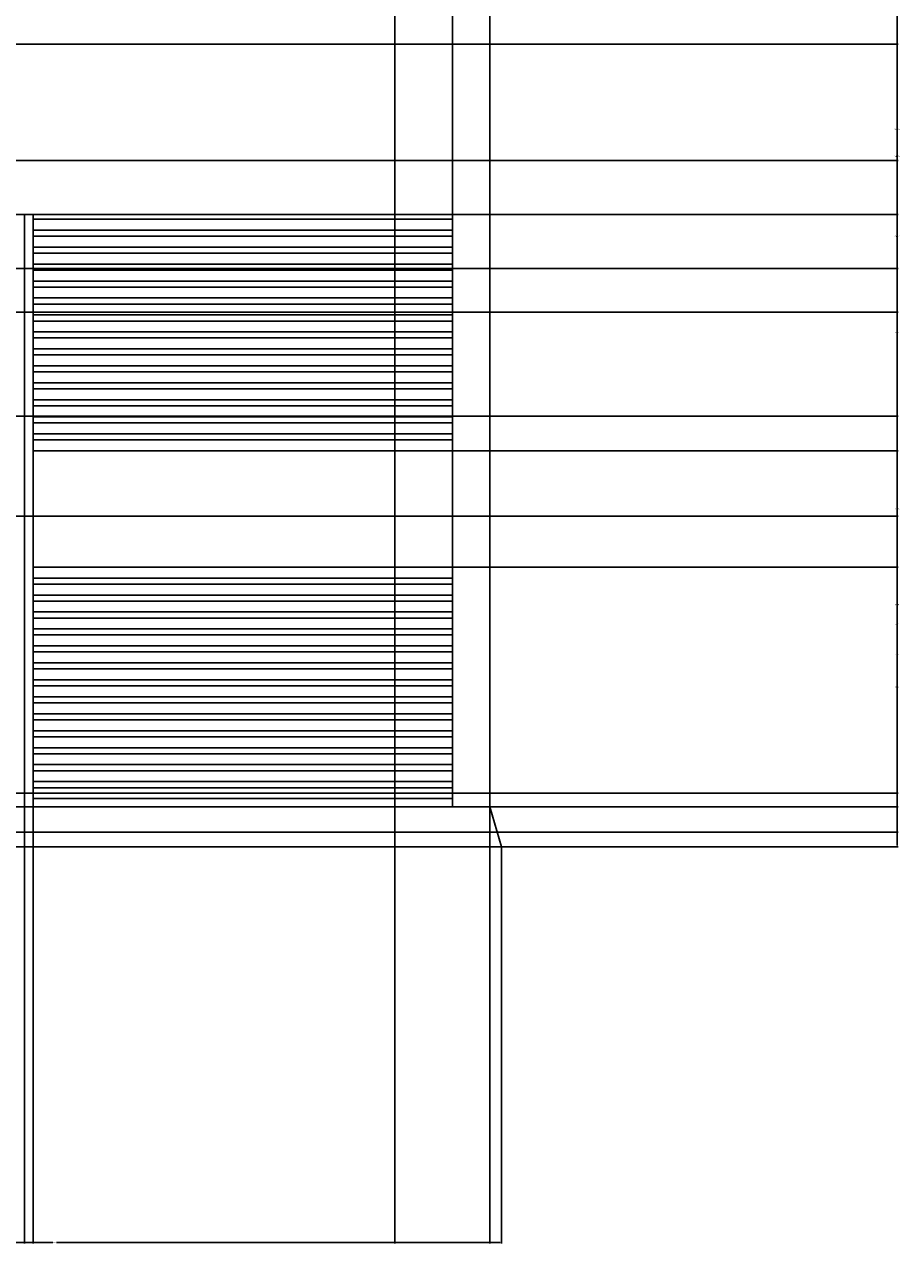
# Model space of a CAD drawing. Units: feet. Extents: x 2193 to 3502, y 890 to 1601.
# Tile 12 of 17: x 3369 to 3502, y 890 to 1076. Entities that reach past the tile are written whole.
import ezdxf

# ---------------------------------------------------------------- set-up
doc = ezdxf.new("R2010")
doc.units = ezdxf.units.FT
doc.layers.add('A-ANNO-DIMS', color=2, linetype='Continuous', lineweight=18)
doc.layers.add('A-ELEV', color=7, linetype='Continuous', lineweight=25)
doc.styles.get("Standard").update_dxf_attribs({"font": 'arial.ttf'})
doc.dimstyles.get("Standard").update_dxf_attribs({"dimtxt": 0.18, "dimasz": 0.18, "dimexe": 0.18, "dimexo": 0.0625, "dimgap": 0.09, "dimtad": 0, "dimtih": 1, "dimtoh": 1, "dimdec": 0, "dimzin": 0, "dimdsep": 46, "dimlunit": 3, "dimtxsty": 'Standard', "dimcen": 0.09, "dimadec": 0, "dimazin": 0, "dimtfac": 1, "dimtdec": 0, "dimtofl": 0, "dimtmove": 0, "dimatfit": 3, "dimfxl": 1, "dimtolj": 1, "dimtzin": 0, "dimarcsym": 0})

# ---------------------------------------------------------------- blocks, each defined once
blk = doc.blocks.new('*D13')
at = {"layer": 'A-ANNO-DIMS', "color": 0, "lineweight": -2, "transparency": 16777216}
for p, q in [((2934.37, 950.89), (2934.37, 1601.47)), ((2934.55, 1601.29), (3186.64, 1601.29)), ((3439.51, 1601.29), (3187.43, 1601.29)), ((3439.69, 1541.11), (3439.69, 1601.47))]:
    blk.add_line(p, q, dxfattribs=at)
at = {"layer": 'A-ANNO-DIMS', "color": 0, "transparency": 16777216}
for points in [[(2934.55, 1601.32), (2934.55, 1601.26), (2934.37, 1601.29)], [(3439.51, 1601.32), (3439.51, 1601.26), (3439.69, 1601.29)]]:
    blk.add_solid(points, dxfattribs=at)
at = {"layer": 'Defpoints', "color": 0, "transparency": 16777216}
for p in [(3439.69, 1601.29), (3439.69, 1541.04), (2934.37, 950.82)]:
    blk.add_point(p, dxfattribs=at)
at = {"layer": 'A-ANNO-DIMS', "color": 0, "transparency": 16777216, "insert": (3187.03, 1601.29), "char_height": 0.18, "attachment_point": 5}
blk.add_mtext('\\A1;505.3', dxfattribs=at)
blk = doc.blocks.new('*D17')
at = {"layer": 'A-ANNO-DIMS', "color": 0, "lineweight": -2, "transparency": 16777216}
for p, q in [((3305.41, 950.76), (3305.41, 890.39)), ((3441.42, 950.76), (3441.42, 890.39)), ((3305.59, 890.57), (3373.14, 890.57)), ((3441.24, 890.57), (3373.7, 890.57))]:
    blk.add_line(p, q, dxfattribs=at)
at = {"layer": 'A-ANNO-DIMS', "color": 0, "transparency": 16777216}
for points in [[(3305.59, 890.6), (3305.59, 890.54), (3305.41, 890.57)], [(3441.24, 890.6), (3441.24, 890.54), (3441.42, 890.57)]]:
    blk.add_solid(points, dxfattribs=at)
at = {"layer": 'Defpoints', "color": 0, "transparency": 16777216}
for p in [(3305.41, 950.82), (3441.42, 950.82), (3441.42, 890.57)]:
    blk.add_point(p, dxfattribs=at)
at = {"layer": 'A-ANNO-DIMS', "color": 0, "transparency": 16777216, "insert": (3373.42, 890.57), "char_height": 0.18, "attachment_point": 5}
blk.add_mtext('\\A1;136', dxfattribs=at)
blk = doc.blocks.new('*D18')
at = {"layer": 'A-ANNO-DIMS', "color": 0, "lineweight": -2, "transparency": 16777216}
for p, q in [((3439.75, 1541.04), (3501.85, 1541.04)), ((3501.67, 1540.86), (3501.67, 1246.12)), ((3501.67, 951), (3501.67, 1245.75)), ((3441.48, 950.82), (3501.85, 950.82))]:
    blk.add_line(p, q, dxfattribs=at)
at = {"layer": 'A-ANNO-DIMS', "color": 0, "transparency": 16777216}
for points in [[(3501.64, 1540.86), (3501.7, 1540.86), (3501.67, 1541.04)], [(3501.64, 951), (3501.7, 951), (3501.67, 950.82)]]:
    blk.add_solid(points, dxfattribs=at)
at = {"layer": 'Defpoints', "color": 0, "transparency": 16777216}
for p in [(3439.69, 1541.04), (3501.67, 1541.04), (3441.42, 950.82)]:
    blk.add_point(p, dxfattribs=at)
at = {"layer": 'A-ANNO-DIMS', "color": 0, "transparency": 16777216, "insert": (3501.67, 1245.93), "char_height": 0.18, "attachment_point": 5}
blk.add_mtext('\\A1;590.2', dxfattribs=at)
blk = doc.blocks.new('*D25')
at = {"layer": 'A-ANNO-DIMS', "color": 0, "lineweight": -2, "transparency": 16777216}
for p, q in [((3070.17, 1073.03), (3501.85, 1073.03)), ((3501.67, 1072.85), (3501.67, 1056.13)), ((3501.67, 1039.05), (3501.67, 1055.77)), ((3067.73, 1038.87), (3501.85, 1038.87))]:
    blk.add_line(p, q, dxfattribs=at)
at = {"layer": 'A-ANNO-DIMS', "color": 0, "transparency": 16777216}
for points in [[(3501.64, 1072.85), (3501.7, 1072.85), (3501.67, 1073.03)], [(3501.64, 1039.05), (3501.7, 1039.05), (3501.67, 1038.87)]]:
    blk.add_solid(points, dxfattribs=at)
at = {"layer": 'Defpoints', "color": 0, "transparency": 16777216}
for p in [(3070.11, 1073.03), (3501.67, 1073.03), (3067.66, 1038.87)]:
    blk.add_point(p, dxfattribs=at)
at = {"layer": 'A-ANNO-DIMS', "color": 0, "transparency": 16777216, "insert": (3501.67, 1055.95), "char_height": 0.18, "attachment_point": 5}
blk.add_mtext('\\A1;34.165', dxfattribs=at)
blk = doc.blocks.new('*D31')
at = {"layer": 'A-ANNO-DIMS', "color": 0, "lineweight": -2, "transparency": 16777216}
for p, q in [((2760.54, 1541.04), (3501.85, 1541.04)), ((3501.67, 1540.86), (3501.67, 1246.12)), ((3501.67, 951), (3501.67, 1245.75)), ((2762.27, 950.82), (3501.85, 950.82))]:
    blk.add_line(p, q, dxfattribs=at)
at = {"layer": 'A-ANNO-DIMS', "color": 0, "transparency": 16777216}
for points in [[(3501.64, 1540.86), (3501.7, 1540.86), (3501.67, 1541.04)], [(3501.64, 951), (3501.7, 951), (3501.67, 950.82)]]:
    blk.add_solid(points, dxfattribs=at)
at = {"layer": 'Defpoints', "color": 0, "transparency": 16777216}
for p in [(2760.47, 1541.04), (3501.67, 1541.04), (2762.2, 950.82)]:
    blk.add_point(p, dxfattribs=at)
at = {"layer": 'A-ANNO-DIMS', "color": 0, "transparency": 16777216, "insert": (3501.67, 1245.93), "char_height": 0.18, "attachment_point": 5}
blk.add_mtext('\\A1;590.2', dxfattribs=at)
blk = doc.blocks.new('*D70')
at = {"layer": 'A-ANNO-DIMS', "color": 0, "lineweight": -2, "transparency": 16777216}
for p, q in [((3425.19, 1166.17), (3425.19, 890.39)), ((3439.69, 1166.17), (3439.69, 890.39)), ((3425.37, 890.57), (3431.98, 890.57)), ((3439.51, 890.57), (3432.89, 890.57))]:
    blk.add_line(p, q, dxfattribs=at)
at = {"layer": 'A-ANNO-DIMS', "color": 0, "transparency": 16777216}
for points in [[(3425.37, 890.6), (3425.37, 890.54), (3425.19, 890.57)], [(3439.51, 890.6), (3439.51, 890.54), (3439.69, 890.57)]]:
    blk.add_solid(points, dxfattribs=at)
at = {"layer": 'Defpoints', "color": 0, "transparency": 16777216}
for p in [(3425.19, 1166.23), (3439.69, 1166.23), (3439.69, 890.57)]:
    blk.add_point(p, dxfattribs=at)
at = {"layer": 'A-ANNO-DIMS', "color": 0, "transparency": 16777216, "insert": (3432.44, 890.57), "char_height": 0.18, "attachment_point": 5}
blk.add_mtext('\\A1;14.502', dxfattribs=at)
blk = doc.blocks.new('*D101')
at = {"layer": 'A-ANNO-DIMS', "color": 0, "lineweight": -2, "transparency": 16777216}
for p, q in [((3265.16, 1055.31), (3501.85, 1055.31)), ((3501.67, 1055.13), (3501.67, 1043.93)), ((3501.67, 1032.37), (3501.67, 1043.57)), ((3265.16, 1032.19), (3501.85, 1032.19))]:
    blk.add_line(p, q, dxfattribs=at)
at = {"layer": 'A-ANNO-DIMS', "color": 0, "transparency": 16777216}
for points in [[(3501.64, 1055.13), (3501.7, 1055.13), (3501.67, 1055.31)], [(3501.64, 1032.37), (3501.7, 1032.37), (3501.67, 1032.19)]]:
    blk.add_solid(points, dxfattribs=at)
at = {"layer": 'Defpoints', "color": 0, "transparency": 16777216}
for p in [(3265.1, 1055.31), (3501.67, 1055.31), (3265.1, 1032.19)]:
    blk.add_point(p, dxfattribs=at)
at = {"layer": 'A-ANNO-DIMS', "color": 0, "transparency": 16777216, "insert": (3501.67, 1043.75), "char_height": 0.18, "attachment_point": 5}
blk.add_mtext('\\A1;23.113', dxfattribs=at)
blk = doc.blocks.new('*D103')
at = {"layer": 'A-ANNO-DIMS', "color": 0, "lineweight": -2, "transparency": 16777216}
for p, q in [((3279.67, 1016.4), (3501.85, 1016.4)), ((3501.67, 1016.22), (3501.67, 984.9)), ((3501.67, 953.21), (3501.67, 984.53)), ((3279.67, 953.03), (3501.85, 953.03))]:
    blk.add_line(p, q, dxfattribs=at)
at = {"layer": 'A-ANNO-DIMS', "color": 0, "transparency": 16777216}
for points in [[(3501.64, 1016.22), (3501.7, 1016.22), (3501.67, 1016.4)], [(3501.64, 953.21), (3501.7, 953.21), (3501.67, 953.03)]]:
    blk.add_solid(points, dxfattribs=at)
at = {"layer": 'Defpoints', "color": 0, "transparency": 16777216}
for p in [(3279.61, 1016.4), (3501.67, 1016.4), (3279.61, 953.03)]:
    blk.add_point(p, dxfattribs=at)
at = {"layer": 'A-ANNO-DIMS', "color": 0, "transparency": 16777216, "insert": (3501.67, 984.72), "char_height": 0.18, "attachment_point": 5}
blk.add_mtext('\\A1;63.37', dxfattribs=at)
blk = doc.blocks.new('*D114')
at = {"layer": 'A-ANNO-DIMS', "color": 0, "lineweight": -2, "transparency": 16777216}
for p, q in [((3157.89, 1001.13), (3501.85, 1001.13)), ((3501.67, 1000.95), (3501.67, 980.23)), ((3501.67, 959.14), (3501.67, 979.86)), ((3159.36, 958.96), (3501.85, 958.96))]:
    blk.add_line(p, q, dxfattribs=at)
at = {"layer": 'A-ANNO-DIMS', "color": 0, "transparency": 16777216}
for points in [[(3501.64, 1000.95), (3501.7, 1000.95), (3501.67, 1001.13)], [(3501.64, 959.14), (3501.7, 959.14), (3501.67, 958.96)]]:
    blk.add_solid(points, dxfattribs=at)
at = {"layer": 'Defpoints', "color": 0, "transparency": 16777216}
for p in [(3157.83, 1001.13), (3501.67, 1001.13), (3159.3, 958.96)]:
    blk.add_point(p, dxfattribs=at)
at = {"layer": 'A-ANNO-DIMS', "color": 0, "transparency": 16777216, "insert": (3501.67, 980.04), "char_height": 0.18, "attachment_point": 5}
blk.add_mtext('\\A1;42.18', dxfattribs=at)
blk = doc.blocks.new('*D115')
at = {"layer": 'A-ANNO-DIMS', "color": 0, "lineweight": -2, "transparency": 16777216}
for p, q in [((3192.61, 1016.4), (3501.85, 1016.4)), ((3501.67, 1016.22), (3501.67, 987.86)), ((3501.67, 959.14), (3501.67, 987.5)), ((3194.2, 958.96), (3501.85, 958.96))]:
    blk.add_line(p, q, dxfattribs=at)
at = {"layer": 'A-ANNO-DIMS', "color": 0, "transparency": 16777216}
for points in [[(3501.64, 1016.22), (3501.7, 1016.22), (3501.67, 1016.4)], [(3501.64, 959.14), (3501.7, 959.14), (3501.67, 958.96)]]:
    blk.add_solid(points, dxfattribs=at)
at = {"layer": 'Defpoints', "color": 0, "transparency": 16777216}
for p in [(3192.55, 1016.4), (3501.67, 1016.4), (3194.13, 958.96)]:
    blk.add_point(p, dxfattribs=at)
at = {"layer": 'A-ANNO-DIMS', "color": 0, "transparency": 16777216, "insert": (3501.67, 987.68), "char_height": 0.18, "attachment_point": 5}
blk.add_mtext('\\A1;57.44', dxfattribs=at)
blk = doc.blocks.new('*D117')
at = {"layer": 'A-ANNO-DIMS', "color": 0, "lineweight": -2, "transparency": 16777216}
for p, q in [((3434.05, 993.39), (3501.85, 993.39)), ((3501.67, 993.21), (3501.67, 975.32)), ((3501.67, 957.06), (3501.67, 974.96)), ((3434.05, 956.88), (3501.85, 956.88))]:
    blk.add_line(p, q, dxfattribs=at)
at = {"layer": 'A-ANNO-DIMS', "color": 0, "transparency": 16777216}
for points in [[(3501.64, 993.21), (3501.7, 993.21), (3501.67, 993.39)], [(3501.64, 957.06), (3501.7, 957.06), (3501.67, 956.88)]]:
    blk.add_solid(points, dxfattribs=at)
at = {"layer": 'Defpoints', "color": 0, "transparency": 16777216}
for p in [(3433.98, 993.39), (3501.67, 993.39), (3433.98, 956.88)]:
    blk.add_point(p, dxfattribs=at)
at = {"layer": 'A-ANNO-DIMS', "color": 0, "transparency": 16777216, "insert": (3501.67, 975.14), "char_height": 0.18, "attachment_point": 5}
blk.add_mtext('\\A1;36.51', dxfattribs=at)
blk = doc.blocks.new('*D118')
at = {"layer": 'A-ANNO-DIMS', "color": 0, "lineweight": -2, "transparency": 16777216}
for p, q in [((3434.05, 1011.12), (3501.85, 1011.12)), ((3501.67, 1010.94), (3501.67, 1002.44)), ((3501.67, 993.57), (3501.67, 1002.08)), ((3434.05, 993.39), (3501.85, 993.39))]:
    blk.add_line(p, q, dxfattribs=at)
at = {"layer": 'A-ANNO-DIMS', "color": 0, "transparency": 16777216}
for points in [[(3501.64, 1010.94), (3501.7, 1010.94), (3501.67, 1011.12)], [(3501.64, 993.57), (3501.7, 993.57), (3501.67, 993.39)]]:
    blk.add_solid(points, dxfattribs=at)
at = {"layer": 'Defpoints', "color": 0, "transparency": 16777216}
for p in [(3433.98, 1011.12), (3501.67, 1011.12), (3433.98, 993.39)]:
    blk.add_point(p, dxfattribs=at)
at = {"layer": 'A-ANNO-DIMS', "color": 0, "transparency": 16777216, "insert": (3501.67, 1002.26), "char_height": 0.18, "attachment_point": 5}
blk.add_mtext('\\A1;17.732', dxfattribs=at)
blk = doc.blocks.new('*D119')
at = {"layer": 'A-ANNO-DIMS', "color": 0, "lineweight": -2, "transparency": 16777216}
for p, q in [((3434.05, 1047.1), (3501.85, 1047.1)), ((3501.67, 1046.92), (3501.67, 1029.29)), ((3501.67, 1011.3), (3501.67, 1028.93)), ((3434.05, 1011.12), (3501.85, 1011.12))]:
    blk.add_line(p, q, dxfattribs=at)
at = {"layer": 'A-ANNO-DIMS', "color": 0, "transparency": 16777216}
for points in [[(3501.64, 1046.92), (3501.7, 1046.92), (3501.67, 1047.1)], [(3501.64, 1011.3), (3501.7, 1011.3), (3501.67, 1011.12)]]:
    blk.add_solid(points, dxfattribs=at)
at = {"layer": 'Defpoints', "color": 0, "transparency": 16777216}
for p in [(3433.98, 1047.1), (3501.67, 1047.1), (3433.98, 1011.12)]:
    blk.add_point(p, dxfattribs=at)
at = {"layer": 'A-ANNO-DIMS', "color": 0, "transparency": 16777216, "insert": (3501.67, 1029.11), "char_height": 0.18, "attachment_point": 5}
blk.add_mtext('\\A1;35.97', dxfattribs=at)
blk = doc.blocks.new('*D120')
at = {"layer": 'A-ANNO-DIMS', "color": 0, "lineweight": -2, "transparency": 16777216}
for p, q in [((3434.05, 1073.03), (3501.85, 1073.03)), ((3501.67, 1072.85), (3501.67, 1060.25)), ((3501.67, 1047.28), (3501.67, 1059.88)), ((3434.05, 1047.1), (3501.85, 1047.1))]:
    blk.add_line(p, q, dxfattribs=at)
at = {"layer": 'A-ANNO-DIMS', "color": 0, "transparency": 16777216}
for points in [[(3501.64, 1072.85), (3501.7, 1072.85), (3501.67, 1073.03)], [(3501.64, 1047.28), (3501.7, 1047.28), (3501.67, 1047.1)]]:
    blk.add_solid(points, dxfattribs=at)
at = {"layer": 'Defpoints', "color": 0, "transparency": 16777216}
for p in [(3433.98, 1073.03), (3501.67, 1073.03), (3433.98, 1047.1)]:
    blk.add_point(p, dxfattribs=at)
at = {"layer": 'A-ANNO-DIMS', "color": 0, "transparency": 16777216, "insert": (3501.67, 1060.06), "char_height": 0.18, "attachment_point": 5}
blk.add_mtext('\\A1;25.935', dxfattribs=at)
blk = doc.blocks.new('*D121')
at = {"layer": 'A-ANNO-DIMS', "color": 0, "lineweight": -2, "transparency": 16777216}
for p, q in [((3304.97, 956.82), (3304.97, 890.39)), ((3368.82, 956.82), (3368.82, 890.39)), ((3305.15, 890.57), (3336.5, 890.57)), ((3368.64, 890.57), (3337.29, 890.57))]:
    blk.add_line(p, q, dxfattribs=at)
at = {"layer": 'A-ANNO-DIMS', "color": 0, "transparency": 16777216}
for points in [[(3305.15, 890.6), (3305.15, 890.54), (3304.97, 890.57)], [(3368.64, 890.6), (3368.64, 890.54), (3368.82, 890.57)]]:
    blk.add_solid(points, dxfattribs=at)
at = {"layer": 'Defpoints', "color": 0, "transparency": 16777216}
for p in [(3304.97, 956.88), (3368.82, 956.88), (3368.82, 890.57)]:
    blk.add_point(p, dxfattribs=at)
at = {"layer": 'A-ANNO-DIMS', "color": 0, "transparency": 16777216, "insert": (3336.9, 890.57), "char_height": 0.18, "attachment_point": 5}
blk.add_mtext('\\A1;63.84', dxfattribs=at)
blk = doc.blocks.new('*D122')
at = {"layer": 'A-ANNO-DIMS', "color": 0, "lineweight": -2, "transparency": 16777216}
for p, q in [((3368.82, 1047.03), (3368.82, 890.39)), ((3370.14, 1047.03), (3370.14, 890.39)), ((3369, 890.57), (3369.16, 890.57)), ((3369.96, 890.57), (3369.79, 890.57))]:
    blk.add_line(p, q, dxfattribs=at)
at = {"layer": 'A-ANNO-DIMS', "color": 0, "transparency": 16777216}
for points in [[(3369, 890.6), (3369, 890.54), (3368.82, 890.57)], [(3369.96, 890.6), (3369.96, 890.54), (3370.14, 890.57)]]:
    blk.add_solid(points, dxfattribs=at)
at = {"layer": 'Defpoints', "color": 0, "transparency": 16777216}
for p in [(3368.82, 1047.1), (3370.14, 1047.1), (3370.14, 890.57)]:
    blk.add_point(p, dxfattribs=at)
at = {"layer": 'A-ANNO-DIMS', "color": 0, "transparency": 16777216, "insert": (3369.48, 890.57), "char_height": 0.18, "attachment_point": 5}
blk.add_mtext('\\A1;1.32', dxfattribs=at)
blk = doc.blocks.new('*D123')
at = {"layer": 'A-ANNO-DIMS', "color": 0, "lineweight": -2, "transparency": 16777216}
for p, q in [((3433.98, 1073.09), (3433.98, 1601.47)), ((3434.16, 1601.29), (3436.44, 1601.29)), ((3439.51, 1601.29), (3437.23, 1601.29)), ((3439.69, 1073.09), (3439.69, 1601.47))]:
    blk.add_line(p, q, dxfattribs=at)
at = {"layer": 'A-ANNO-DIMS', "color": 0, "transparency": 16777216}
for points in [[(3434.16, 1601.32), (3434.16, 1601.26), (3433.98, 1601.29)], [(3439.51, 1601.32), (3439.51, 1601.26), (3439.69, 1601.29)]]:
    blk.add_solid(points, dxfattribs=at)
at = {"layer": 'Defpoints', "color": 0, "transparency": 16777216}
for p in [(3439.69, 1601.29), (3433.98, 1073.03), (3439.69, 1073.03)]:
    blk.add_point(p, dxfattribs=at)
at = {"layer": 'A-ANNO-DIMS', "color": 0, "transparency": 16777216, "insert": (3436.84, 1601.29), "char_height": 0.18, "attachment_point": 5}
blk.add_mtext('\\A1;5.707', dxfattribs=at)

msp = doc.modelspace()

# ---------------------------------------------------------------- linework, layer by layer
at = {"layer": 'A-ELEV'}
for p, q in [((3439.6901, 956.8829), (3439.6901, 1494.0584)), ((2934.3742, 1073.031), (3439.6901, 1073.031)), ((3439.6901, 956.8829), (3441.4216, 950.8228)), ((3305.4139, 950.8228), (3441.4216, 950.8228))]:
    msp.add_line(p, q, dxfattribs=at)
for points in [[(3439.6901, 1073.031), (3439.6901, 956.8829), (3433.9829, 956.8829), (3433.9829, 1073.031)], [(3368.8176, 956.8829), (3368.8176, 1047.0961), (3370.1383, 1047.0961), (3370.1383, 956.8829)], [(3370.1383, 1046.365), (3433.9829, 1046.365), (3433.9829, 1044.7027), (3370.1383, 1044.7027)], [(3370.1383, 1043.7821), (3433.9829, 1043.7821), (3433.9829, 1042.1198), (3370.1383, 1042.1198)], [(3370.1383, 1041.1991), (3433.9829, 1041.1991), (3433.9829, 1039.5368), (3370.1383, 1039.5368)], [(3370.1383, 1038.6162), (3433.9829, 1038.6162), (3433.9829, 1036.9539), (3370.1383, 1036.9539)], [(3370.1383, 1036.0333), (3433.9829, 1036.0333), (3433.9829, 1034.371), (3370.1383, 1034.371)], [(3370.1383, 1033.4503), (3433.9829, 1033.4503), (3433.9829, 1031.788), (3370.1383, 1031.788)], [(3370.1383, 1030.8674), (3433.9829, 1030.8674), (3433.9829, 1029.2051), (3370.1383, 1029.2051)], [(3370.1383, 1028.2844), (3433.9829, 1028.2844), (3433.9829, 1026.6222), (3370.1383, 1026.6222)], [(3370.1383, 1025.7015), (3433.9829, 1025.7015), (3433.9829, 1024.0392), (3370.1383, 1024.0392)], [(3370.1383, 1023.1186), (3433.9829, 1023.1186), (3433.9829, 1021.4563), (3370.1383, 1021.4563)], [(3370.1383, 1020.5356), (3433.9829, 1020.5356), (3433.9829, 1018.8734), (3370.1383, 1018.8734)], [(3370.1383, 1017.9527), (3433.9829, 1017.9527), (3433.9829, 1016.2904), (3370.1383, 1016.2904)], [(3370.1383, 1015.3698), (3433.9829, 1015.3698), (3433.9829, 1013.7075), (3370.1383, 1013.7075)], [(3370.1383, 1012.7868), (3433.9829, 1012.7868), (3433.9829, 1011.1246), (3370.1383, 1011.1246)], [(3370.1383, 993.3923), (3433.9829, 993.3923), (3433.9829, 991.7301), (3370.1383, 991.7301)], [(3370.1383, 990.8094), (3433.9829, 990.8094), (3433.9829, 989.1471), (3370.1383, 989.1471)], [(3370.1383, 988.2265), (3433.9829, 988.2265), (3433.9829, 986.5642), (3370.1383, 986.5642)], [(3370.1383, 985.6435), (3433.9829, 985.6435), (3433.9829, 983.9813), (3370.1383, 983.9813)], [(3370.1383, 983.0606), (3433.9829, 983.0606), (3433.9829, 981.3983), (3370.1383, 981.3983)], [(3370.1383, 980.4777), (3433.9829, 980.4777), (3433.9829, 978.8154), (3370.1383, 978.8154)], [(3370.1383, 977.8947), (3433.9829, 977.8947), (3433.9829, 976.2325), (3370.1383, 976.2325)], [(3370.1383, 975.3118), (3433.9829, 975.3118), (3433.9829, 973.6495), (3370.1383, 973.6495)], [(3370.1383, 972.7289), (3433.9829, 972.7289), (3433.9829, 971.0666), (3370.1383, 971.0666)], [(3370.1383, 970.1459), (3433.9829, 970.1459), (3433.9829, 968.4837), (3370.1383, 968.4837)], [(3370.1383, 967.563), (3433.9829, 967.563), (3433.9829, 965.9007), (3370.1383, 965.9007)], [(3370.1383, 964.9801), (3433.9829, 964.9801), (3433.9829, 963.3178), (3370.1383, 963.3178)], [(3370.1383, 962.3971), (3433.9829, 962.3971), (3433.9829, 960.7348), (3370.1383, 960.7348)], [(3370.1383, 959.8142), (3433.9829, 959.8142), (3433.9829, 958.1519), (3370.1383, 958.1519)]]:
    msp.add_lwpolyline(points, dxfattribs=at)
msp.add_lwpolyline([(3433.9829, 956.8829), (3304.9731, 956.8829), (3304.9731, 1047.0961), (3433.9829, 1047.0961)], close=True, dxfattribs=at)

# ---------------------------------------------------------------- dimensions: what is measured, and where the dimension line sits
at = {"layer": 'A-ANNO-DIMS'}
for base, p1, p2, override, picture, middle in [((3439.6901, 1601.2941), (2934.3742, 950.8228), (3439.6901, 1541.0441), {"dimdec": 1, "dimlfac": 1, "dimrnd": 0, "dimzin": 0, "dimdsep": 46, "dimlunit": 2}, '*D13', (3187.0321, 1601.2941)), ((3439.6901, 1601.2941), (3433.9829, 1073.031), (3439.6901, 1073.031), {"dimdec": 3, "dimlfac": 1, "dimrnd": 0, "dimzin": 0, "dimdsep": 46, "dimlunit": 2}, '*D123', (3436.8365, 1601.2941)), ((3439.6901, 890.5728), (3425.1877, 1166.2327), (3439.6901, 1166.2327), {"dimdec": 3, "dimlfac": 1, "dimrnd": 0, "dimzin": 0, "dimdsep": 46, "dimlunit": 2}, '*D70', (3432.4389, 890.5728)), ((3370.1383, 890.5728), (3368.8176, 1047.0961), (3370.1383, 1047.0961), {"dimdec": 2, "dimlfac": 1, "dimrnd": 0, "dimzin": 0, "dimdsep": 46, "dimlunit": 2}, '*D122', (3369.478, 890.5728)), ((3368.8176, 890.5728), (3304.9731, 956.8829), (3368.8176, 956.8829), {"dimdec": 2, "dimlfac": 1, "dimrnd": 0, "dimzin": 0, "dimdsep": 46, "dimlunit": 2}, '*D121', (3336.8953, 890.5728)), ((3441.4216, 890.5728), (3305.4139, 950.8228), (3441.4216, 950.8228), {"dimdec": 0, "dimlfac": 1, "dimrnd": 0, "dimzin": 0, "dimdsep": 46, "dimlunit": 2}, '*D17', (3373.4177, 890.5728))]:
    dim = msp.add_linear_dim(base=base, p1=p1, p2=p2, dimstyle='Standard', override=override, dxfattribs=at)
    dim.commit()
    dim.dimension.update_dxf_attribs({"geometry": picture, "text_midpoint": middle})
for base, p1, p2, override, picture, middle in [((3501.6716, 1541.0441), (2762.2048, 950.8228), (2760.4733, 1541.0441), {"dimdec": 1, "dimlfac": 1, "dimrnd": 0, "dimzin": 0, "dimdsep": 46, "dimlunit": 2}, '*D31', (3501.6716, 1245.9334)), ((3501.6716, 1541.0441), (3441.4216, 950.8228), (3439.6901, 1541.0441), {"dimdec": 1, "dimlfac": 1, "dimrnd": 0, "dimzin": 0, "dimdsep": 46, "dimlunit": 2}, '*D18', (3501.6716, 1245.9334)), ((3501.6716, 1073.031), (3067.665, 1038.8658), (3070.1101, 1073.031), {"dimdec": 3, "dimlfac": 1, "dimrnd": 0, "dimzin": 0, "dimdsep": 46, "dimlunit": 2}, '*D25', (3501.6716, 1055.9484)), ((3501.6716, 1073.031), (3433.9829, 1047.0961), (3433.9829, 1073.031), {"dimdec": 3, "dimlfac": 1, "dimrnd": 0, "dimzin": 0, "dimdsep": 46, "dimlunit": 2}, '*D120', (3501.6716, 1060.0636)), ((3501.6716, 1055.3069), (3265.1012, 1032.1935), (3265.1012, 1055.3069), {"dimdec": 3, "dimlfac": 1, "dimrnd": 0, "dimzin": 0, "dimdsep": 46, "dimlunit": 2}, '*D101', (3501.6716, 1043.7502)), ((3501.6716, 1047.0961), (3433.9829, 1011.1246), (3433.9829, 1047.0961), {"dimdec": 2, "dimlfac": 1, "dimrnd": 0, "dimzin": 0, "dimdsep": 46, "dimlunit": 2}, '*D119', (3501.6716, 1029.1103)), ((3501.6716, 1016.4), (3194.1338, 958.9555), (3192.5464, 1016.4), {"dimdec": 2, "dimlfac": 1, "dimrnd": 0, "dimzin": 0, "dimdsep": 46, "dimlunit": 2}, '*D115', (3501.6716, 987.6777)), ((3501.6716, 1016.4), (3279.6085, 953.031), (3279.6085, 1016.4), {"dimdec": 2, "dimlfac": 1, "dimrnd": 0, "dimzin": 0, "dimdsep": 46, "dimlunit": 2}, '*D103', (3501.6716, 984.7155)), ((3501.6716, 1011.1246), (3433.9829, 993.3923), (3433.9829, 1011.1246), {"dimdec": 3, "dimlfac": 1, "dimrnd": 0, "dimzin": 0, "dimdsep": 46, "dimlunit": 2}, '*D118', (3501.6716, 1002.2584)), ((3501.6716, 1001.1334), (3159.2977, 958.9555), (3157.8263, 1001.1334), {"dimdec": 2, "dimlfac": 1, "dimrnd": 0, "dimzin": 0, "dimdsep": 46, "dimlunit": 2}, '*D114', (3501.6716, 980.0444)), ((3501.6716, 993.3923), (3433.9829, 956.8829), (3433.9829, 993.3923), {"dimdec": 2, "dimlfac": 1, "dimrnd": 0, "dimzin": 0, "dimdsep": 46, "dimlunit": 2}, '*D117', (3501.6716, 975.1376))]:
    dim = msp.add_linear_dim(base=base, p1=p1, p2=p2, angle=90, dimstyle='Standard', override=override, dxfattribs=at)
    dim.commit()
    dim.dimension.update_dxf_attribs({"geometry": picture, "text_midpoint": middle})

doc.saveas('drawing.dxf')
